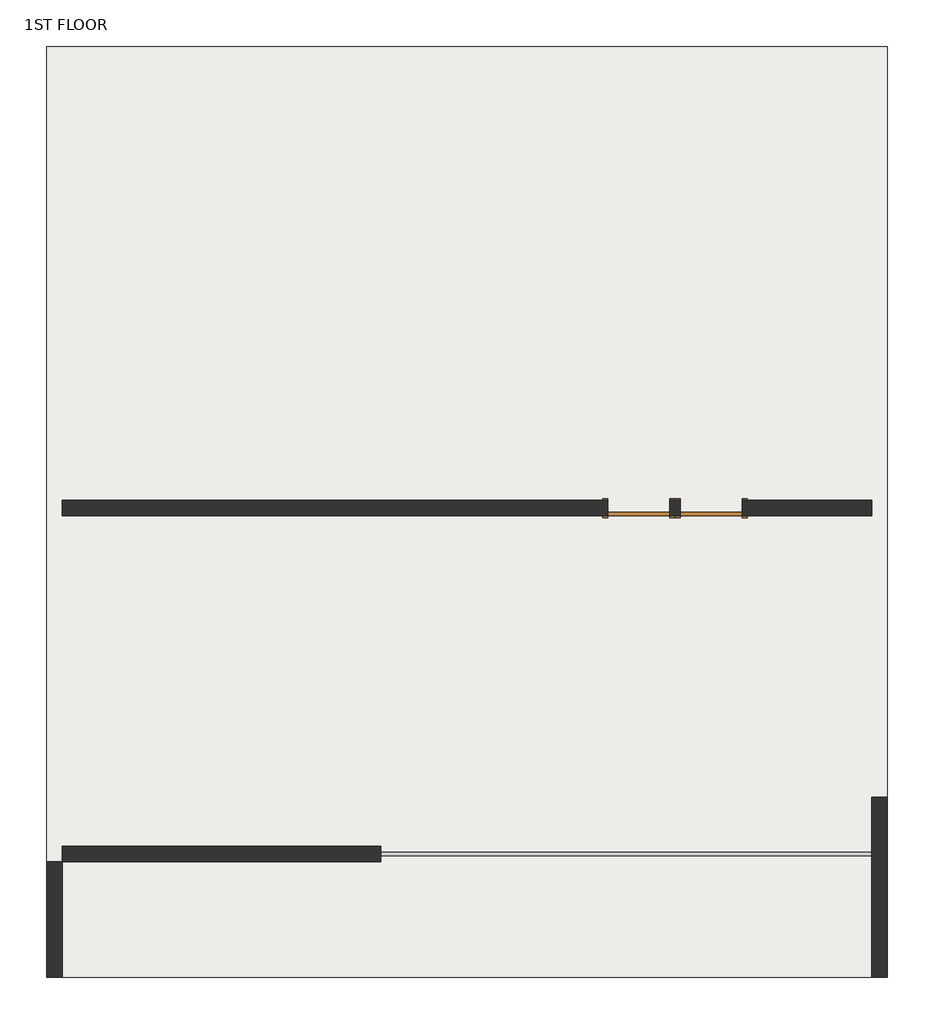
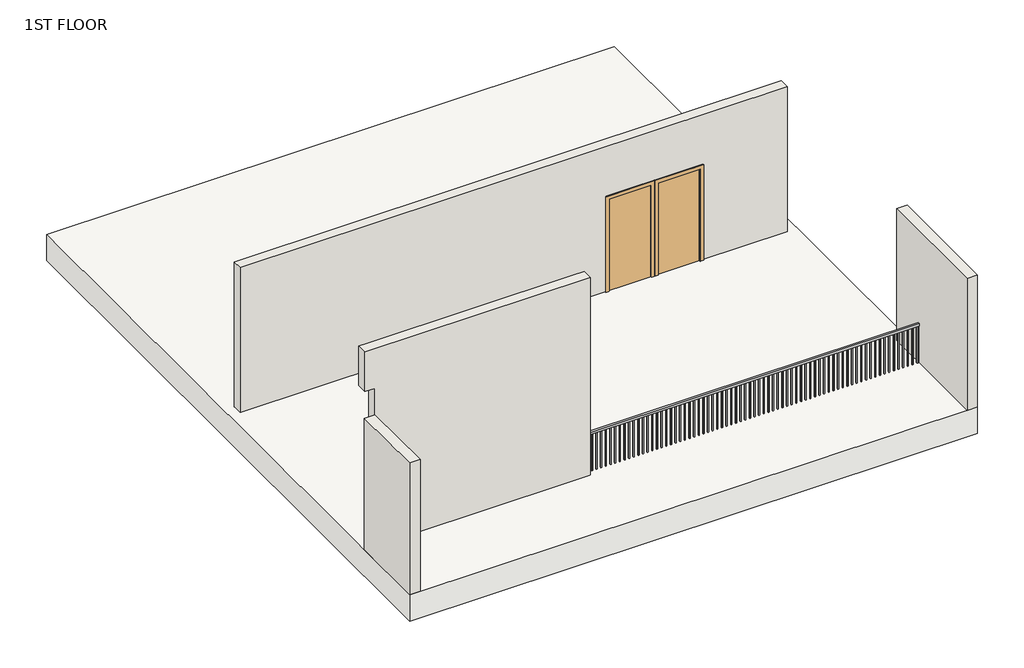
# One storey: 4 walls, 2 doors, 1 railing, 1 slab.
"""IFC4 building model written with IfcOpenShell, lengths in millimetres."""

from ifc_helpers import new_model, si_unit, frame, origin, place, context, project, spatial, polyline, outline, extrude, faceted_brep, transform, mapped, element, save
from components import door_0ca8825f

model = new_model("IFC4")

# Units and contexts
model_context = context("Model", 3, world=origin())
ifc_project = project(units=[si_unit("LENGTHUNIT", "METRE", prefix="MILLI")], contexts=[model_context])

# Site, building, storey
site = spatial("IfcSite", under=ifc_project)
building = spatial("IfcBuilding", under=site)
storey = spatial("IfcBuildingStorey", under=building, Name="1ST FLOOR", Elevation=3352.8)

# Doors
placement = place(None, origin())
door_shape = door_0ca8825f(model_context)
element("IfcDoor", 1, ObjectType="Single-Flush : 36\" x 84\"", at=placement, inside=storey, context=model_context, shape_type="MappedRepresentation", body=[
    mapped(door_shape, transform((-4413.6008651, 6628.7047421, 3352.8), x_axis=(-1.0, 0.0, 0.0), y_axis=(0.0, -1.0, 0.0), z_axis=(0.0, 0.0, 1.0))),
])
element("IfcDoor", 2, ObjectType="Single-Flush : 36\" x 84\"", at=placement, inside=storey, context=model_context, shape_type="MappedRepresentation", body=[
    mapped(door_shape, transform((-3346.8008651, 6628.7047421, 3352.8), x_axis=(-1.0, 0.0, 0.0), y_axis=(0.0, -1.0, 0.0), z_axis=(0.0, 0.0, 1.0))),
])

# Railing
element("IfcRailing", 3, ObjectType="Handrail - Rectangular", at=placement, inside=storey, context=model_context, shape_type="SweptSolid", body=[
    extrude(outline(polyline([(-8223.6008651, 1497.9047421), (-8223.6008651, 1548.7047421), (-971.9008651, 1548.7047421), (-971.9008651, 1497.9047421), (-8223.6008651, 1497.9047421)])), frame((0.0, 0.0, 4216.4), z_axis=(0.0, 0.0, 1.0), x_axis=(1.0, 0.0, 0.0)), (0.0, 0.0, 1.0), 50.8),
    extrude(outline(polyline([(-1019.5258651, 1513.7797421), (-1019.5258651, 1532.8297421), (-1000.4758651, 1532.8297421), (-1000.4758651, 1513.7797421), (-1019.5258651, 1513.7797421)])), frame((0.0, 0.0, 3352.8), z_axis=(0.0, 0.0, 1.0), x_axis=(1.0, 0.0, 0.0)), (0.0, 0.0, 1.0), 863.6),
    extrude(outline(polyline([(-1121.1258651, 1513.7797421), (-1121.1258651, 1532.8297421), (-1102.0758651, 1532.8297421), (-1102.0758651, 1513.7797421), (-1121.1258651, 1513.7797421)])), frame((0.0, 0.0, 3352.8), z_axis=(0.0, 0.0, 1.0), x_axis=(1.0, 0.0, 0.0)), (0.0, 0.0, 1.0), 863.6),
    extrude(outline(polyline([(-1222.7258651, 1513.7797421), (-1222.7258651, 1532.8297421), (-1203.6758651, 1532.8297421), (-1203.6758651, 1513.7797421), (-1222.7258651, 1513.7797421)])), frame((0.0, 0.0, 3352.8), z_axis=(0.0, 0.0, 1.0), x_axis=(1.0, 0.0, 0.0)), (0.0, 0.0, 1.0), 863.6),
    extrude(outline(polyline([(-1324.3258651, 1513.7797421), (-1324.3258651, 1532.8297421), (-1305.2758651, 1532.8297421), (-1305.2758651, 1513.7797421), (-1324.3258651, 1513.7797421)])), frame((0.0, 0.0, 3352.8), z_axis=(0.0, 0.0, 1.0), x_axis=(1.0, 0.0, 0.0)), (0.0, 0.0, 1.0), 863.6),
    extrude(outline(polyline([(-1425.9258651, 1513.7797421), (-1425.9258651, 1532.8297421), (-1406.8758651, 1532.8297421), (-1406.8758651, 1513.7797421), (-1425.9258651, 1513.7797421)])), frame((0.0, 0.0, 3352.8), z_axis=(0.0, 0.0, 1.0), x_axis=(1.0, 0.0, 0.0)), (0.0, 0.0, 1.0), 863.6),
    extrude(outline(polyline([(-1527.5258651, 1513.7797421), (-1527.5258651, 1532.8297421), (-1508.4758651, 1532.8297421), (-1508.4758651, 1513.7797421), (-1527.5258651, 1513.7797421)])), frame((0.0, 0.0, 3352.8), z_axis=(0.0, 0.0, 1.0), x_axis=(1.0, 0.0, 0.0)), (0.0, 0.0, 1.0), 863.6),
    extrude(outline(polyline([(-1629.1258651, 1513.7797421), (-1629.1258651, 1532.8297421), (-1610.0758651, 1532.8297421), (-1610.0758651, 1513.7797421), (-1629.1258651, 1513.7797421)])), frame((0.0, 0.0, 3352.8), z_axis=(0.0, 0.0, 1.0), x_axis=(1.0, 0.0, 0.0)), (0.0, 0.0, 1.0), 863.6),
    extrude(outline(polyline([(-1730.7258651, 1513.7797421), (-1730.7258651, 1532.8297421), (-1711.6758651, 1532.8297421), (-1711.6758651, 1513.7797421), (-1730.7258651, 1513.7797421)])), frame((0.0, 0.0, 3352.8), z_axis=(0.0, 0.0, 1.0), x_axis=(1.0, 0.0, 0.0)), (0.0, 0.0, 1.0), 863.6),
    extrude(outline(polyline([(-1832.3258651, 1513.7797421), (-1832.3258651, 1532.8297421), (-1813.2758651, 1532.8297421), (-1813.2758651, 1513.7797421), (-1832.3258651, 1513.7797421)])), frame((0.0, 0.0, 3352.8), z_axis=(0.0, 0.0, 1.0), x_axis=(1.0, 0.0, 0.0)), (0.0, 0.0, 1.0), 863.6),
    extrude(outline(polyline([(-1933.9258651, 1513.7797421), (-1933.9258651, 1532.8297421), (-1914.8758651, 1532.8297421), (-1914.8758651, 1513.7797421), (-1933.9258651, 1513.7797421)])), frame((0.0, 0.0, 3352.8), z_axis=(0.0, 0.0, 1.0), x_axis=(1.0, 0.0, 0.0)), (0.0, 0.0, 1.0), 863.6),
    extrude(outline(polyline([(-2035.5258651, 1513.7797421), (-2035.5258651, 1532.8297421), (-2016.4758651, 1532.8297421), (-2016.4758651, 1513.7797421), (-2035.5258651, 1513.7797421)])), frame((0.0, 0.0, 3352.8), z_axis=(0.0, 0.0, 1.0), x_axis=(1.0, 0.0, 0.0)), (0.0, 0.0, 1.0), 863.6),
    extrude(outline(polyline([(-2137.1258651, 1513.7797421), (-2137.1258651, 1532.8297421), (-2118.0758651, 1532.8297421), (-2118.0758651, 1513.7797421), (-2137.1258651, 1513.7797421)])), frame((0.0, 0.0, 3352.8), z_axis=(0.0, 0.0, 1.0), x_axis=(1.0, 0.0, 0.0)), (0.0, 0.0, 1.0), 863.6),
    extrude(outline(polyline([(-2238.7258651, 1513.7797421), (-2238.7258651, 1532.8297421), (-2219.6758651, 1532.8297421), (-2219.6758651, 1513.7797421), (-2238.7258651, 1513.7797421)])), frame((0.0, 0.0, 3352.8), z_axis=(0.0, 0.0, 1.0), x_axis=(1.0, 0.0, 0.0)), (0.0, 0.0, 1.0), 863.6),
    extrude(outline(polyline([(-2340.3258651, 1513.7797421), (-2340.3258651, 1532.8297421), (-2321.2758651, 1532.8297421), (-2321.2758651, 1513.7797421), (-2340.3258651, 1513.7797421)])), frame((0.0, 0.0, 3352.8), z_axis=(0.0, 0.0, 1.0), x_axis=(1.0, 0.0, 0.0)), (0.0, 0.0, 1.0), 863.6),
    extrude(outline(polyline([(-2441.9258651, 1513.7797421), (-2441.9258651, 1532.8297421), (-2422.8758651, 1532.8297421), (-2422.8758651, 1513.7797421), (-2441.9258651, 1513.7797421)])), frame((0.0, 0.0, 3352.8), z_axis=(0.0, 0.0, 1.0), x_axis=(1.0, 0.0, 0.0)), (0.0, 0.0, 1.0), 863.6),
    extrude(outline(polyline([(-2543.5258651, 1513.7797421), (-2543.5258651, 1532.8297421), (-2524.4758651, 1532.8297421), (-2524.4758651, 1513.7797421), (-2543.5258651, 1513.7797421)])), frame((0.0, 0.0, 3352.8), z_axis=(0.0, 0.0, 1.0), x_axis=(1.0, 0.0, 0.0)), (0.0, 0.0, 1.0), 863.6),
    extrude(outline(polyline([(-2645.1258651, 1513.7797421), (-2645.1258651, 1532.8297421), (-2626.0758651, 1532.8297421), (-2626.0758651, 1513.7797421), (-2645.1258651, 1513.7797421)])), frame((0.0, 0.0, 3352.8), z_axis=(0.0, 0.0, 1.0), x_axis=(1.0, 0.0, 0.0)), (0.0, 0.0, 1.0), 863.6),
    extrude(outline(polyline([(-2746.7258651, 1513.7797421), (-2746.7258651, 1532.8297421), (-2727.6758651, 1532.8297421), (-2727.6758651, 1513.7797421), (-2746.7258651, 1513.7797421)])), frame((0.0, 0.0, 3352.8), z_axis=(0.0, 0.0, 1.0), x_axis=(1.0, 0.0, 0.0)), (0.0, 0.0, 1.0), 863.6),
    extrude(outline(polyline([(-2848.3258651, 1513.7797421), (-2848.3258651, 1532.8297421), (-2829.2758651, 1532.8297421), (-2829.2758651, 1513.7797421), (-2848.3258651, 1513.7797421)])), frame((0.0, 0.0, 3352.8), z_axis=(0.0, 0.0, 1.0), x_axis=(1.0, 0.0, 0.0)), (0.0, 0.0, 1.0), 863.6),
    extrude(outline(polyline([(-2949.9258651, 1513.7797421), (-2949.9258651, 1532.8297421), (-2930.8758651, 1532.8297421), (-2930.8758651, 1513.7797421), (-2949.9258651, 1513.7797421)])), frame((0.0, 0.0, 3352.8), z_axis=(0.0, 0.0, 1.0), x_axis=(1.0, 0.0, 0.0)), (0.0, 0.0, 1.0), 863.6),
    extrude(outline(polyline([(-3051.5258651, 1513.7797421), (-3051.5258651, 1532.8297421), (-3032.4758651, 1532.8297421), (-3032.4758651, 1513.7797421), (-3051.5258651, 1513.7797421)])), frame((0.0, 0.0, 3352.8), z_axis=(0.0, 0.0, 1.0), x_axis=(1.0, 0.0, 0.0)), (0.0, 0.0, 1.0), 863.6),
    extrude(outline(polyline([(-3153.1258651, 1513.7797421), (-3153.1258651, 1532.8297421), (-3134.0758651, 1532.8297421), (-3134.0758651, 1513.7797421), (-3153.1258651, 1513.7797421)])), frame((0.0, 0.0, 3352.8), z_axis=(0.0, 0.0, 1.0), x_axis=(1.0, 0.0, 0.0)), (0.0, 0.0, 1.0), 863.6),
    extrude(outline(polyline([(-3254.7258651, 1513.7797421), (-3254.7258651, 1532.8297421), (-3235.6758651, 1532.8297421), (-3235.6758651, 1513.7797421), (-3254.7258651, 1513.7797421)])), frame((0.0, 0.0, 3352.8), z_axis=(0.0, 0.0, 1.0), x_axis=(1.0, 0.0, 0.0)), (0.0, 0.0, 1.0), 863.6),
    extrude(outline(polyline([(-3356.3258651, 1513.7797421), (-3356.3258651, 1532.8297421), (-3337.2758651, 1532.8297421), (-3337.2758651, 1513.7797421), (-3356.3258651, 1513.7797421)])), frame((0.0, 0.0, 3352.8), z_axis=(0.0, 0.0, 1.0), x_axis=(1.0, 0.0, 0.0)), (0.0, 0.0, 1.0), 863.6),
    extrude(outline(polyline([(-3457.9258651, 1513.7797421), (-3457.9258651, 1532.8297421), (-3438.8758651, 1532.8297421), (-3438.8758651, 1513.7797421), (-3457.9258651, 1513.7797421)])), frame((0.0, 0.0, 3352.8), z_axis=(0.0, 0.0, 1.0), x_axis=(1.0, 0.0, 0.0)), (0.0, 0.0, 1.0), 863.6),
    extrude(outline(polyline([(-3559.5258651, 1513.7797421), (-3559.5258651, 1532.8297421), (-3540.4758651, 1532.8297421), (-3540.4758651, 1513.7797421), (-3559.5258651, 1513.7797421)])), frame((0.0, 0.0, 3352.8), z_axis=(0.0, 0.0, 1.0), x_axis=(1.0, 0.0, 0.0)), (0.0, 0.0, 1.0), 863.6),
    extrude(outline(polyline([(-3661.1258651, 1513.7797421), (-3661.1258651, 1532.8297421), (-3642.0758651, 1532.8297421), (-3642.0758651, 1513.7797421), (-3661.1258651, 1513.7797421)])), frame((0.0, 0.0, 3352.8), z_axis=(0.0, 0.0, 1.0), x_axis=(1.0, 0.0, 0.0)), (0.0, 0.0, 1.0), 863.6),
    extrude(outline(polyline([(-3762.7258651, 1513.7797421), (-3762.7258651, 1532.8297421), (-3743.6758651, 1532.8297421), (-3743.6758651, 1513.7797421), (-3762.7258651, 1513.7797421)])), frame((0.0, 0.0, 3352.8), z_axis=(0.0, 0.0, 1.0), x_axis=(1.0, 0.0, 0.0)), (0.0, 0.0, 1.0), 863.6),
    extrude(outline(polyline([(-3864.3258651, 1513.7797421), (-3864.3258651, 1532.8297421), (-3845.2758651, 1532.8297421), (-3845.2758651, 1513.7797421), (-3864.3258651, 1513.7797421)])), frame((0.0, 0.0, 3352.8), z_axis=(0.0, 0.0, 1.0), x_axis=(1.0, 0.0, 0.0)), (0.0, 0.0, 1.0), 863.6),
    extrude(outline(polyline([(-3965.9258651, 1513.7797421), (-3965.9258651, 1532.8297421), (-3946.8758651, 1532.8297421), (-3946.8758651, 1513.7797421), (-3965.9258651, 1513.7797421)])), frame((0.0, 0.0, 3352.8), z_axis=(0.0, 0.0, 1.0), x_axis=(1.0, 0.0, 0.0)), (0.0, 0.0, 1.0), 863.6),
    extrude(outline(polyline([(-4067.5258651, 1513.7797421), (-4067.5258651, 1532.8297421), (-4048.4758651, 1532.8297421), (-4048.4758651, 1513.7797421), (-4067.5258651, 1513.7797421)])), frame((0.0, 0.0, 3352.8), z_axis=(0.0, 0.0, 1.0), x_axis=(1.0, 0.0, 0.0)), (0.0, 0.0, 1.0), 863.6),
    extrude(outline(polyline([(-4169.1258651, 1513.7797421), (-4169.1258651, 1532.8297421), (-4150.0758651, 1532.8297421), (-4150.0758651, 1513.7797421), (-4169.1258651, 1513.7797421)])), frame((0.0, 0.0, 3352.8), z_axis=(0.0, 0.0, 1.0), x_axis=(1.0, 0.0, 0.0)), (0.0, 0.0, 1.0), 863.6),
    extrude(outline(polyline([(-4270.7258651, 1513.7797421), (-4270.7258651, 1532.8297421), (-4251.6758651, 1532.8297421), (-4251.6758651, 1513.7797421), (-4270.7258651, 1513.7797421)])), frame((0.0, 0.0, 3352.8), z_axis=(0.0, 0.0, 1.0), x_axis=(1.0, 0.0, 0.0)), (0.0, 0.0, 1.0), 863.6),
    extrude(outline(polyline([(-4372.3258651, 1513.7797421), (-4372.3258651, 1532.8297421), (-4353.2758651, 1532.8297421), (-4353.2758651, 1513.7797421), (-4372.3258651, 1513.7797421)])), frame((0.0, 0.0, 3352.8), z_axis=(0.0, 0.0, 1.0), x_axis=(1.0, 0.0, 0.0)), (0.0, 0.0, 1.0), 863.6),
    extrude(outline(polyline([(-4473.9258651, 1513.7797421), (-4473.9258651, 1532.8297421), (-4454.8758651, 1532.8297421), (-4454.8758651, 1513.7797421), (-4473.9258651, 1513.7797421)])), frame((0.0, 0.0, 3352.8), z_axis=(0.0, 0.0, 1.0), x_axis=(1.0, 0.0, 0.0)), (0.0, 0.0, 1.0), 863.6),
    extrude(outline(polyline([(-4575.5258651, 1513.7797421), (-4575.5258651, 1532.8297421), (-4556.4758651, 1532.8297421), (-4556.4758651, 1513.7797421), (-4575.5258651, 1513.7797421)])), frame((0.0, 0.0, 3352.8), z_axis=(0.0, 0.0, 1.0), x_axis=(1.0, 0.0, 0.0)), (0.0, 0.0, 1.0), 863.6),
    extrude(outline(polyline([(-4677.1258651, 1513.7797421), (-4677.1258651, 1532.8297421), (-4658.0758651, 1532.8297421), (-4658.0758651, 1513.7797421), (-4677.1258651, 1513.7797421)])), frame((0.0, 0.0, 3352.8), z_axis=(0.0, 0.0, 1.0), x_axis=(1.0, 0.0, 0.0)), (0.0, 0.0, 1.0), 863.6),
    extrude(outline(polyline([(-4778.7258651, 1513.7797421), (-4778.7258651, 1532.8297421), (-4759.6758651, 1532.8297421), (-4759.6758651, 1513.7797421), (-4778.7258651, 1513.7797421)])), frame((0.0, 0.0, 3352.8), z_axis=(0.0, 0.0, 1.0), x_axis=(1.0, 0.0, 0.0)), (0.0, 0.0, 1.0), 863.6),
    extrude(outline(polyline([(-4880.3258651, 1513.7797421), (-4880.3258651, 1532.8297421), (-4861.2758651, 1532.8297421), (-4861.2758651, 1513.7797421), (-4880.3258651, 1513.7797421)])), frame((0.0, 0.0, 3352.8), z_axis=(0.0, 0.0, 1.0), x_axis=(1.0, 0.0, 0.0)), (0.0, 0.0, 1.0), 863.6),
    extrude(outline(polyline([(-4981.9258651, 1513.7797421), (-4981.9258651, 1532.8297421), (-4962.8758651, 1532.8297421), (-4962.8758651, 1513.7797421), (-4981.9258651, 1513.7797421)])), frame((0.0, 0.0, 3352.8), z_axis=(0.0, 0.0, 1.0), x_axis=(1.0, 0.0, 0.0)), (0.0, 0.0, 1.0), 863.6),
    extrude(outline(polyline([(-5083.5258651, 1513.7797421), (-5083.5258651, 1532.8297421), (-5064.4758651, 1532.8297421), (-5064.4758651, 1513.7797421), (-5083.5258651, 1513.7797421)])), frame((0.0, 0.0, 3352.8), z_axis=(0.0, 0.0, 1.0), x_axis=(1.0, 0.0, 0.0)), (0.0, 0.0, 1.0), 863.6),
    extrude(outline(polyline([(-5185.1258651, 1513.7797421), (-5185.1258651, 1532.8297421), (-5166.0758651, 1532.8297421), (-5166.0758651, 1513.7797421), (-5185.1258651, 1513.7797421)])), frame((0.0, 0.0, 3352.8), z_axis=(0.0, 0.0, 1.0), x_axis=(1.0, 0.0, 0.0)), (0.0, 0.0, 1.0), 863.6),
    extrude(outline(polyline([(-5286.7258651, 1513.7797421), (-5286.7258651, 1532.8297421), (-5267.6758651, 1532.8297421), (-5267.6758651, 1513.7797421), (-5286.7258651, 1513.7797421)])), frame((0.0, 0.0, 3352.8), z_axis=(0.0, 0.0, 1.0), x_axis=(1.0, 0.0, 0.0)), (0.0, 0.0, 1.0), 863.6),
    extrude(outline(polyline([(-5388.3258651, 1513.7797421), (-5388.3258651, 1532.8297421), (-5369.2758651, 1532.8297421), (-5369.2758651, 1513.7797421), (-5388.3258651, 1513.7797421)])), frame((0.0, 0.0, 3352.8), z_axis=(0.0, 0.0, 1.0), x_axis=(1.0, 0.0, 0.0)), (0.0, 0.0, 1.0), 863.6),
    extrude(outline(polyline([(-5489.9258651, 1513.7797421), (-5489.9258651, 1532.8297421), (-5470.8758651, 1532.8297421), (-5470.8758651, 1513.7797421), (-5489.9258651, 1513.7797421)])), frame((0.0, 0.0, 3352.8), z_axis=(0.0, 0.0, 1.0), x_axis=(1.0, 0.0, 0.0)), (0.0, 0.0, 1.0), 863.6),
    extrude(outline(polyline([(-5591.5258651, 1513.7797421), (-5591.5258651, 1532.8297421), (-5572.4758651, 1532.8297421), (-5572.4758651, 1513.7797421), (-5591.5258651, 1513.7797421)])), frame((0.0, 0.0, 3352.8), z_axis=(0.0, 0.0, 1.0), x_axis=(1.0, 0.0, 0.0)), (0.0, 0.0, 1.0), 863.6),
    extrude(outline(polyline([(-5693.1258651, 1513.7797421), (-5693.1258651, 1532.8297421), (-5674.0758651, 1532.8297421), (-5674.0758651, 1513.7797421), (-5693.1258651, 1513.7797421)])), frame((0.0, 0.0, 3352.8), z_axis=(0.0, 0.0, 1.0), x_axis=(1.0, 0.0, 0.0)), (0.0, 0.0, 1.0), 863.6),
    extrude(outline(polyline([(-5794.7258651, 1513.7797421), (-5794.7258651, 1532.8297421), (-5775.6758651, 1532.8297421), (-5775.6758651, 1513.7797421), (-5794.7258651, 1513.7797421)])), frame((0.0, 0.0, 3352.8), z_axis=(0.0, 0.0, 1.0), x_axis=(1.0, 0.0, 0.0)), (0.0, 0.0, 1.0), 863.6),
    extrude(outline(polyline([(-5896.3258651, 1513.7797421), (-5896.3258651, 1532.8297421), (-5877.2758651, 1532.8297421), (-5877.2758651, 1513.7797421), (-5896.3258651, 1513.7797421)])), frame((0.0, 0.0, 3352.8), z_axis=(0.0, 0.0, 1.0), x_axis=(1.0, 0.0, 0.0)), (0.0, 0.0, 1.0), 863.6),
    extrude(outline(polyline([(-5997.9258651, 1513.7797421), (-5997.9258651, 1532.8297421), (-5978.8758651, 1532.8297421), (-5978.8758651, 1513.7797421), (-5997.9258651, 1513.7797421)])), frame((0.0, 0.0, 3352.8), z_axis=(0.0, 0.0, 1.0), x_axis=(1.0, 0.0, 0.0)), (0.0, 0.0, 1.0), 863.6),
    extrude(outline(polyline([(-6099.5258651, 1513.7797421), (-6099.5258651, 1532.8297421), (-6080.4758651, 1532.8297421), (-6080.4758651, 1513.7797421), (-6099.5258651, 1513.7797421)])), frame((0.0, 0.0, 3352.8), z_axis=(0.0, 0.0, 1.0), x_axis=(1.0, 0.0, 0.0)), (0.0, 0.0, 1.0), 863.6),
    extrude(outline(polyline([(-6201.1258651, 1513.7797421), (-6201.1258651, 1532.8297421), (-6182.0758651, 1532.8297421), (-6182.0758651, 1513.7797421), (-6201.1258651, 1513.7797421)])), frame((0.0, 0.0, 3352.8), z_axis=(0.0, 0.0, 1.0), x_axis=(1.0, 0.0, 0.0)), (0.0, 0.0, 1.0), 863.6),
    extrude(outline(polyline([(-6302.7258651, 1513.7797421), (-6302.7258651, 1532.8297421), (-6283.6758651, 1532.8297421), (-6283.6758651, 1513.7797421), (-6302.7258651, 1513.7797421)])), frame((0.0, 0.0, 3352.8), z_axis=(0.0, 0.0, 1.0), x_axis=(1.0, 0.0, 0.0)), (0.0, 0.0, 1.0), 863.6),
    extrude(outline(polyline([(-6404.3258651, 1513.7797421), (-6404.3258651, 1532.8297421), (-6385.2758651, 1532.8297421), (-6385.2758651, 1513.7797421), (-6404.3258651, 1513.7797421)])), frame((0.0, 0.0, 3352.8), z_axis=(0.0, 0.0, 1.0), x_axis=(1.0, 0.0, 0.0)), (0.0, 0.0, 1.0), 863.6),
    extrude(outline(polyline([(-6505.9258651, 1513.7797421), (-6505.9258651, 1532.8297421), (-6486.8758651, 1532.8297421), (-6486.8758651, 1513.7797421), (-6505.9258651, 1513.7797421)])), frame((0.0, 0.0, 3352.8), z_axis=(0.0, 0.0, 1.0), x_axis=(1.0, 0.0, 0.0)), (0.0, 0.0, 1.0), 863.6),
    extrude(outline(polyline([(-6607.5258651, 1513.7797421), (-6607.5258651, 1532.8297421), (-6588.4758651, 1532.8297421), (-6588.4758651, 1513.7797421), (-6607.5258651, 1513.7797421)])), frame((0.0, 0.0, 3352.8), z_axis=(0.0, 0.0, 1.0), x_axis=(1.0, 0.0, 0.0)), (0.0, 0.0, 1.0), 863.6),
    extrude(outline(polyline([(-6709.1258651, 1513.7797421), (-6709.1258651, 1532.8297421), (-6690.0758651, 1532.8297421), (-6690.0758651, 1513.7797421), (-6709.1258651, 1513.7797421)])), frame((0.0, 0.0, 3352.8), z_axis=(0.0, 0.0, 1.0), x_axis=(1.0, 0.0, 0.0)), (0.0, 0.0, 1.0), 863.6),
    extrude(outline(polyline([(-6810.7258651, 1513.7797421), (-6810.7258651, 1532.8297421), (-6791.6758651, 1532.8297421), (-6791.6758651, 1513.7797421), (-6810.7258651, 1513.7797421)])), frame((0.0, 0.0, 3352.8), z_axis=(0.0, 0.0, 1.0), x_axis=(1.0, 0.0, 0.0)), (0.0, 0.0, 1.0), 863.6),
    extrude(outline(polyline([(-6912.3258651, 1513.7797421), (-6912.3258651, 1532.8297421), (-6893.2758651, 1532.8297421), (-6893.2758651, 1513.7797421), (-6912.3258651, 1513.7797421)])), frame((0.0, 0.0, 3352.8), z_axis=(0.0, 0.0, 1.0), x_axis=(1.0, 0.0, 0.0)), (0.0, 0.0, 1.0), 863.6),
    extrude(outline(polyline([(-7013.9258651, 1513.7797421), (-7013.9258651, 1532.8297421), (-6994.8758651, 1532.8297421), (-6994.8758651, 1513.7797421), (-7013.9258651, 1513.7797421)])), frame((0.0, 0.0, 3352.8), z_axis=(0.0, 0.0, 1.0), x_axis=(1.0, 0.0, 0.0)), (0.0, 0.0, 1.0), 863.6),
    extrude(outline(polyline([(-7115.5258651, 1513.7797421), (-7115.5258651, 1532.8297421), (-7096.4758651, 1532.8297421), (-7096.4758651, 1513.7797421), (-7115.5258651, 1513.7797421)])), frame((0.0, 0.0, 3352.8), z_axis=(0.0, 0.0, 1.0), x_axis=(1.0, 0.0, 0.0)), (0.0, 0.0, 1.0), 863.6),
    extrude(outline(polyline([(-7217.1258651, 1513.7797421), (-7217.1258651, 1532.8297421), (-7198.0758651, 1532.8297421), (-7198.0758651, 1513.7797421), (-7217.1258651, 1513.7797421)])), frame((0.0, 0.0, 3352.8), z_axis=(0.0, 0.0, 1.0), x_axis=(1.0, 0.0, 0.0)), (0.0, 0.0, 1.0), 863.6),
    extrude(outline(polyline([(-7318.7258651, 1513.7797421), (-7318.7258651, 1532.8297421), (-7299.6758651, 1532.8297421), (-7299.6758651, 1513.7797421), (-7318.7258651, 1513.7797421)])), frame((0.0, 0.0, 3352.8), z_axis=(0.0, 0.0, 1.0), x_axis=(1.0, 0.0, 0.0)), (0.0, 0.0, 1.0), 863.6),
    extrude(outline(polyline([(-7420.3258651, 1513.7797421), (-7420.3258651, 1532.8297421), (-7401.2758651, 1532.8297421), (-7401.2758651, 1513.7797421), (-7420.3258651, 1513.7797421)])), frame((0.0, 0.0, 3352.8), z_axis=(0.0, 0.0, 1.0), x_axis=(1.0, 0.0, 0.0)), (0.0, 0.0, 1.0), 863.6),
    extrude(outline(polyline([(-7521.9258651, 1513.7797421), (-7521.9258651, 1532.8297421), (-7502.8758651, 1532.8297421), (-7502.8758651, 1513.7797421), (-7521.9258651, 1513.7797421)])), frame((0.0, 0.0, 3352.8), z_axis=(0.0, 0.0, 1.0), x_axis=(1.0, 0.0, 0.0)), (0.0, 0.0, 1.0), 863.6),
    extrude(outline(polyline([(-7623.5258651, 1513.7797421), (-7623.5258651, 1532.8297421), (-7604.4758651, 1532.8297421), (-7604.4758651, 1513.7797421), (-7623.5258651, 1513.7797421)])), frame((0.0, 0.0, 3352.8), z_axis=(0.0, 0.0, 1.0), x_axis=(1.0, 0.0, 0.0)), (0.0, 0.0, 1.0), 863.6),
    extrude(outline(polyline([(-7725.1258651, 1513.7797421), (-7725.1258651, 1532.8297421), (-7706.0758651, 1532.8297421), (-7706.0758651, 1513.7797421), (-7725.1258651, 1513.7797421)])), frame((0.0, 0.0, 3352.8), z_axis=(0.0, 0.0, 1.0), x_axis=(1.0, 0.0, 0.0)), (0.0, 0.0, 1.0), 863.6),
    extrude(outline(polyline([(-7826.7258651, 1513.7797421), (-7826.7258651, 1532.8297421), (-7807.6758651, 1532.8297421), (-7807.6758651, 1513.7797421), (-7826.7258651, 1513.7797421)])), frame((0.0, 0.0, 3352.8), z_axis=(0.0, 0.0, 1.0), x_axis=(1.0, 0.0, 0.0)), (0.0, 0.0, 1.0), 863.6),
    extrude(outline(polyline([(-7928.3258651, 1513.7797421), (-7928.3258651, 1532.8297421), (-7909.2758651, 1532.8297421), (-7909.2758651, 1513.7797421), (-7928.3258651, 1513.7797421)])), frame((0.0, 0.0, 3352.8), z_axis=(0.0, 0.0, 1.0), x_axis=(1.0, 0.0, 0.0)), (0.0, 0.0, 1.0), 863.6),
    extrude(outline(polyline([(-8029.9258651, 1513.7797421), (-8029.9258651, 1532.8297421), (-8010.8758651, 1532.8297421), (-8010.8758651, 1513.7797421), (-8029.9258651, 1513.7797421)])), frame((0.0, 0.0, 3352.8), z_axis=(0.0, 0.0, 1.0), x_axis=(1.0, 0.0, 0.0)), (0.0, 0.0, 1.0), 863.6),
    extrude(outline(polyline([(-8131.5258651, 1513.7797421), (-8131.5258651, 1532.8297421), (-8112.4758651, 1532.8297421), (-8112.4758651, 1513.7797421), (-8131.5258651, 1513.7797421)])), frame((0.0, 0.0, 3352.8), z_axis=(0.0, 0.0, 1.0), x_axis=(1.0, 0.0, 0.0)), (0.0, 0.0, 1.0), 863.6),
    extrude(outline(polyline([(-990.9508651, 1513.7797421), (-990.9508651, 1532.8297421), (-971.9008651, 1532.8297421), (-971.9008651, 1513.7797421), (-990.9508651, 1513.7797421)])), frame((0.0, 0.0, 3352.8), z_axis=(0.0, 0.0, 1.0), x_axis=(1.0, 0.0, 0.0)), (0.0, 0.0, 1.0), 863.6),
    extrude(outline(polyline([(-8223.6008651, 1513.7797421), (-8223.6008651, 1532.8297421), (-8204.5508651, 1532.8297421), (-8204.5508651, 1513.7797421), (-8223.6008651, 1513.7797421)])), frame((0.0, 0.0, 3352.8), z_axis=(0.0, 0.0, 1.0), x_axis=(1.0, 0.0, 0.0)), (0.0, 0.0, 1.0), 863.6),
])

# Slab
element("IfcSlab", 4, ObjectType="Generic - 12\"", at=placement, inside=storey, context=model_context, shape_type="SweptSolid", body=[
    extrude(outline(polyline([(-743.3008651, 13448.6047421), (-743.3008651, -303.1418232), (-13163.9008651, -303.1418232), (-13163.9008651, 13448.6047421), (-743.3008651, 13448.6047421)])), frame((0.0, 0.0, 2743.2), z_axis=(0.0, 0.0, 1.0), x_axis=(1.0, 0.0, 0.0)), (0.0, 0.0, 1.0), 609.6),
])

# Walls
element("IfcWall", 5, ObjectType="OTR WALL", at=placement, inside=storey, context=model_context, shape_type="SweptSolid", body=[
    extrude(outline(polyline([(3352.8, -3956.4008651), (3352.8, -3804.0008651), (5486.4, -3804.0008651), (5486.4, -2889.6008651), (3352.8, -2889.6008651), (3352.8, -971.9008651), (6705.6, -971.9008651), (6705.6, -12935.3008651), (3352.8, -12935.3008651), (3352.8, -4870.8008651), (5486.4, -4870.8008651), (5486.4, -3956.4008651), (3352.8, -3956.4008651)])), frame((0.0, 6514.4047421, 0.0), z_axis=(0.0, 1.0, 0.0), x_axis=(0.0, 0.0, 1.0)), (0.0, 0.0, 1.0), 228.6),
])
element("IfcWall", 6, ObjectType="OTR WALL", at=placement, inside=storey, context=model_context, shape_type="Brep", body=[
    faceted_brep([(-12935.3008651, 1409.0047421, 7010.4), (-12935.3008651, 1409.0047421, 6705.6), (-12935.3008651, 1409.0047421, 3352.8), (-8223.6008651, 1409.0047421, 3352.8), (-8223.6008651, 1409.0047421, 7924.8), (-13151.2008651, 1409.0047421, 7924.8), (-13151.2008651, 1409.0047421, 7010.4), (-12935.3008651, 1637.6047421, 3352.8), (-12935.3008651, 1637.6047421, 7010.4), (-12948.0008651, 1637.6047421, 7010.4), (-13151.2008651, 1637.6047421, 7010.4), (-13151.2008651, 1637.6047421, 7924.8), (-12948.0008651, 1637.6047421, 7924.8), (-8426.8008651, 1637.6047421, 7924.8), (-8223.6008651, 1637.6047421, 7924.8), (-8223.6008651, 1637.6047421, 7010.4), (-8223.6008651, 1637.6047421, 3352.8), (-12935.3008651, 1421.7047421, 3352.8)], [[[0, 1, 2, 3, 4, 5, 6]], [[7, 8, 9, 10, 11, 12, 13, 14, 15, 16]], [[3, 2, 17, 7, 16]], [[4, 3, 16, 15, 14]], [[6, 10, 9, 8, 0]], [[0, 8, 7, 17, 2, 1]], [[6, 5, 11, 10]], [[5, 4, 14, 13, 12, 11]]]),
])
element("IfcWall", 7, ObjectType="OTR WALL", at=placement, inside=storey, context=model_context, shape_type="SweptSolid", body=[
    extrude(outline(polyline([(-13163.9008651, -303.1418232), (-13163.9008651, 1409.0047421), (-12935.3008651, 1409.0047421), (-12935.3008651, -303.1418232), (-13163.9008651, -303.1418232)])), frame((0.0, 0.0, 3352.8), z_axis=(0.0, 0.0, 1.0), x_axis=(1.0, 0.0, 0.0)), (0.0, 0.0, 1.0), 3048.0),
])
element("IfcWall", 8, ObjectType="OTR WALL", at=placement, inside=storey, context=model_context, shape_type="SweptSolid", body=[
    extrude(outline(polyline([(-971.9008651, -303.1418232), (-971.9008651, 2361.5047421), (-743.3008651, 2361.5047421), (-743.3008651, -303.1418232), (-971.9008651, -303.1418232)])), frame((0.0, 0.0, 3352.8), z_axis=(0.0, 0.0, 1.0), x_axis=(1.0, 0.0, 0.0)), (0.0, 0.0, 1.0), 3048.0),
])

save(model, "model.ifc")

# Revit data of these elements
# Type "Single-Flush : 36\" x 84\""
#   Type Mark = "1"
#   Construction Type Id = "MDOOR"
#   Assembly Code = "C1020"
#   Analytic Construction = "Metal"
#   Thickness = 0' - 2"
#   Heat Transfer Coefficient (U) = 0.651978 BTU/(h·ft²·°F)
#   Height = 7' - 0"
#   Trim Projection Ext = 0' - 1"
#   Trim Projection Int = 0' - 1"
#   Trim Width = 0' - 3"
#   Width = 3' - 0"
#   Define Thermal Properties by = 1
#   Door Material = Door - Panel
#   Frame Material = Door - Frame
#   Visual Light Transmittance = 0
#   Solar Heat Gain Coefficient = 0
#   Function = (empty or 0)
#   Wall Closure = (empty or 0)
# Type "Handrail - Rectangular"
#   Assembly Code = "C2010400"
#   built-in parameter 1008612 = 0.0416667 (stored number, unit not read)
#   built-in parameter 1008611 = 0.0416667 (stored number, unit not read)
#   built-in parameter 1008609 = 0.333333 (stored number, unit not read)
#   built-in parameter 1008604 = 0.166667 (stored number, unit not read)
#   built-in parameter 1008603 = 0.166667 (stored number, unit not read)
#   Railing Height = 3' - 0"
#   built-in parameter 1008630 = 2
#   built-in parameter 1008610 = 2
#   built-in parameter 1008618 = Baluster - Square : 3/4"
# Type "Generic - 12\""
#   Assembly Code = "B1010"
#   Function = 0
#   Layers, outside or top first: 2' - 0" "Gypsum Wall Board" (function 1)
# Type "OTR WALL"
#   Assembly Code = "B2010"
#   Layers, outside or top first: 0' - 9" "WHITE" (function 1)
# Elements 1, 2 (IfcDoor, "Single-Flush : 36\" x 84\"")
#   Phase Created = New Construction
#   Materials on its faces: "Door - Frame", "Door - Panel"
# Element 3 (IfcRailing, "Handrail - Rectangular")
#   Phase Created = New Construction
# Element 4 (IfcSlab, "Generic - 12\"")
#   Height Offset From Level = 0' - 0"
#   Phase Created = New Construction
#   Materials on its faces: "Gypsum Wall Board"
# Element 5 (IfcWall, "OTR WALL")
#   Top Offset = 0' - 0"
#   Base Offset = 0' - 0"
#   Unconnected Height = 11' - 0"
#   wall height = 11' - 0"
#   Phase Created = New Construction
#   Base Constraint = 1ST FLOOR
#   Materials on its faces: "WHITE"
# Element 6 (IfcWall, "OTR WALL")
#   Top Offset = 0' - 0"
#   Base Offset = 0' - 0"
#   Unconnected Height = 17' - 0"
#   wall height = 17' - 0"
#   Phase Created = New Construction
#   Base Constraint = 1ST FLOOR
#   Materials on its faces: "WHITE", "Default New Material(1)"
# Elements 7, 8 (IfcWall, "OTR WALL")
#   Top Offset = 0' - 0"
#   Base Offset = 0' - 0"
#   Unconnected Height = 10' - 0"
#   wall height = 10' - 0"
#   Phase Created = New Construction
#   Base Constraint = 1ST FLOOR
#   Materials on its faces: "WHITE"
# Materials
#   "Door - Panel": class "Wood", colour RGB 210 159 95, transparency 0
#   "Door - Frame": colour RGB 118 70 51, transparency 0
#   "Gypsum Wall Board": class "Generic", colour RGB 127 127 127, transparency 0, Description = "Gypsum Wall Board", Cost = 0
#   "WHITE": class "Generic", colour RGB 255 255 255, transparency 0, Cost = 0
#   "Default New Material(1)": class "Generic", colour RGB 192 192 192, transparency 0, Cost = 0
